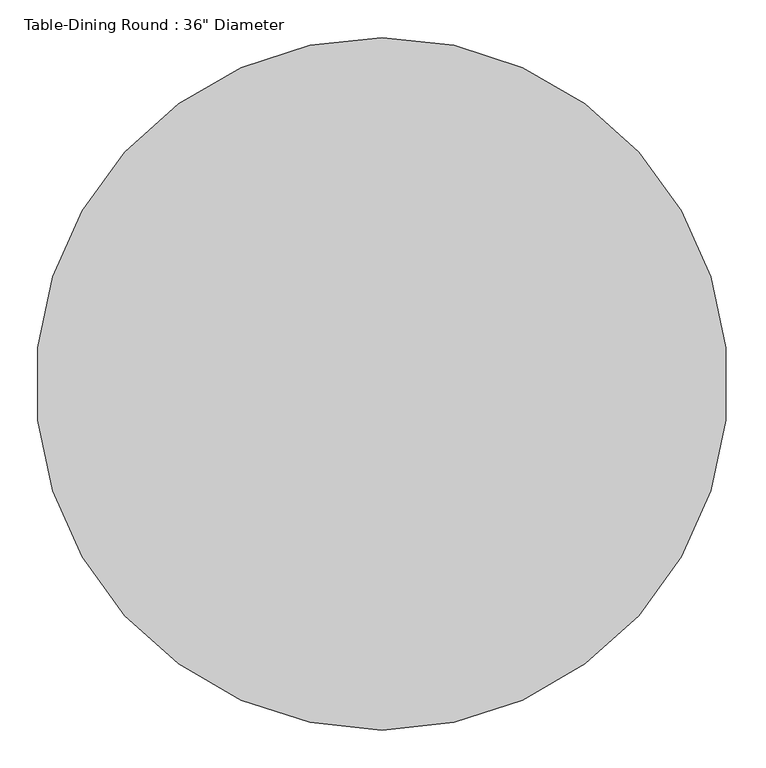
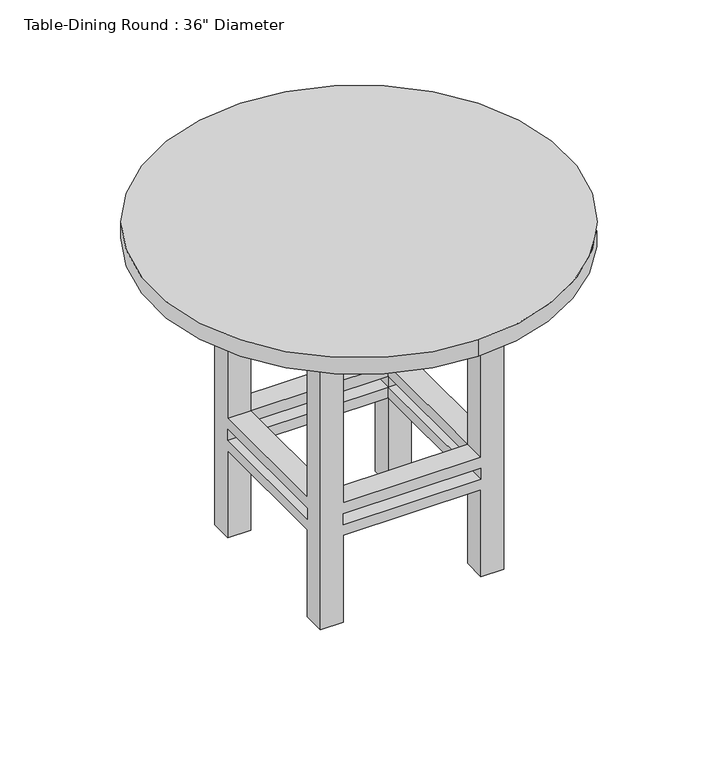
"""IFC4 building model written with IfcOpenShell, lengths in millimetres: furniture geometry."""

from ifc_helpers import new_model, si_unit, point, frame, frame_2d, origin, place, context, project, spatial, polyline, circle_curve, trimmed, segment, composite_curve, outline, extrude, faceted_brep, source, transform, mapped, element, save


def furniture_ec754799(model_context):
    return source(origin(), model_context, "Body", "SolidModel", [
        extrude(outline(polyline([(332.2819672, 43.7213115), (332.2819672, -413.4786885), (-124.9180328, -413.4786885), (-124.9180328, 43.7213115), (332.2819672, 43.7213115)]), holes=[polyline([(306.8819672, 18.3213115), (-99.5180328, 18.3213115), (-99.5180328, -388.0786885), (306.8819672, -388.0786885), (306.8819672, 18.3213115)])]), frame((0.0, 0.0, 647.7), z_axis=(0.0, 0.0, 1.0), x_axis=(1.0, 0.0, 0.0)), (0.0, 0.0, 1.0), 76.2),
        faceted_brep([(-48.7180328, 18.3213115, 723.9), (-99.5180328, 18.3213115, 723.9), (-99.5180328, -32.4786885, 723.9), (-48.7180328, -32.4786885, 723.9), (256.0819672, 18.3213115, 723.9), (256.0819672, -32.4786885, 723.9), (306.8819672, -32.4786885, 723.9), (306.8819672, 18.3213115, 723.9), (256.0819672, -388.0786885, 723.9), (306.8819672, -388.0786885, 723.9), (306.8819672, -337.2786885, 723.9), (256.0819672, -337.2786885, 723.9), (-48.7180328, -388.0786885, 723.9), (-48.7180328, -337.2786885, 723.9), (-99.5180328, -337.2786885, 723.9), (-99.5180328, -388.0786885, 723.9), (-48.7180328, 18.3213115, 0.0), (-48.7180328, -32.4786885, 0.0), (-99.5180328, -32.4786885, 0.0), (-99.5180328, 18.3213115, 0.0), (256.0819672, 18.3213115, 0.0), (306.8819672, 18.3213115, 0.0), (306.8819672, -32.4786885, 0.0), (256.0819672, -32.4786885, 0.0), (256.0819672, -388.0786885, 0.0), (256.0819672, -337.2786885, 0.0), (306.8819672, -337.2786885, 0.0), (306.8819672, -388.0786885, 0.0), (-48.7180328, -388.0786885, 0.0), (-99.5180328, -388.0786885, 0.0), (-99.5180328, -337.2786885, 0.0), (-48.7180328, -337.2786885, 0.0), (-48.7180328, 18.3213115, 279.4), (256.0819672, 18.3213115, 279.4), (256.0819672, 18.3213115, 203.2), (-48.7180328, 18.3213115, 203.2), (256.0819672, 18.3213115, 228.6), (256.0819672, 18.3213115, 254.0), (-48.7180328, 18.3213115, 254.0), (-48.7180328, 18.3213115, 228.6), (-99.5180328, -32.4786885, 203.2), (-99.5180328, -337.2786885, 203.2), (-99.5180328, -337.2786885, 279.4), (-99.5180328, -32.4786885, 279.4), (-99.5180328, -32.4786885, 228.6), (-99.5180328, -32.4786885, 254.0), (-99.5180328, -337.2786885, 254.0), (-99.5180328, -337.2786885, 228.6), (-48.7180328, -32.4786885, 279.4), (-48.7180328, -32.4786885, 203.2), (-48.7180328, -32.4786885, 228.6), (-48.7180328, -32.4786885, 254.0), (256.0819672, -32.4786885, 279.4), (256.0819672, -32.4786885, 203.2), (256.0819672, -32.4786885, 228.6), (256.0819672, -32.4786885, 254.0), (306.8819672, -32.4786885, 279.4), (306.8819672, -32.4786885, 203.2), (306.8819672, -32.4786885, 228.6), (306.8819672, -32.4786885, 254.0), (306.8819672, -337.2786885, 279.4), (306.8819672, -337.2786885, 203.2), (306.8819672, -337.2786885, 228.6), (306.8819672, -337.2786885, 254.0), (256.0819672, -388.0786885, 279.4), (-48.7180328, -388.0786885, 279.4), (-48.7180328, -388.0786885, 203.2), (256.0819672, -388.0786885, 203.2), (-48.7180328, -388.0786885, 228.6), (-48.7180328, -388.0786885, 254.0), (256.0819672, -388.0786885, 254.0), (256.0819672, -388.0786885, 228.6), (256.0819672, -337.2786885, 279.4), (256.0819672, -337.2786885, 203.2), (256.0819672, -337.2786885, 228.6), (256.0819672, -337.2786885, 254.0), (-48.7180328, -337.2786885, 279.4), (-48.7180328, -337.2786885, 203.2), (-48.7180328, -337.2786885, 228.6), (-48.7180328, -337.2786885, 254.0)], [[[0, 1, 2, 3]], [[4, 5, 6, 7]], [[8, 9, 10, 11]], [[12, 13, 14, 15]], [[16, 17, 18, 19]], [[20, 21, 22, 23]], [[24, 25, 26, 27]], [[28, 29, 30, 31]], [[1, 0, 32, 33, 4, 7, 21, 20, 34, 35, 16, 19], [36, 37, 38, 39]], [[2, 1, 19, 18, 40, 41, 30, 29, 15, 14, 42, 43], [44, 45, 46, 47]], [[3, 2, 43, 48]], [[18, 17, 49, 40]], [[44, 50, 51, 45]], [[0, 3, 48, 32]], [[17, 16, 35, 49]], [[50, 39, 38, 51]], [[5, 4, 33, 52]], [[20, 23, 53, 34]], [[36, 54, 55, 37]], [[6, 5, 52, 56]], [[23, 22, 57, 53]], [[54, 58, 59, 55]], [[21, 7, 6, 56, 60, 10, 9, 27, 26, 61, 57, 22], [62, 63, 59, 58]], [[27, 9, 8, 64, 65, 12, 15, 29, 28, 66, 67, 24], [68, 69, 70, 71]], [[11, 10, 60, 72]], [[26, 25, 73, 61]], [[62, 74, 75, 63]], [[8, 11, 72, 64]], [[25, 24, 67, 73]], [[74, 71, 70, 75]], [[13, 12, 65, 76]], [[28, 31, 77, 66]], [[68, 78, 79, 69]], [[14, 13, 76, 42]], [[31, 30, 41, 77]], [[78, 47, 46, 79]], [[54, 74, 62, 58]], [[74, 78, 68, 71]], [[78, 50, 44, 47]], [[50, 54, 36, 39]], [[53, 49, 35, 34]], [[49, 77, 41, 40]], [[77, 73, 67, 66]], [[73, 53, 57, 61]], [[74, 54, 53, 73]], [[78, 74, 73, 77]], [[50, 78, 77, 49]], [[54, 50, 49, 53]], [[52, 72, 60, 56]], [[72, 76, 65, 64]], [[76, 48, 43, 42]], [[48, 52, 33, 32]], [[55, 51, 38, 37]], [[51, 79, 46, 45]], [[79, 75, 70, 69]], [[75, 55, 59, 63]], [[72, 52, 55, 75]], [[76, 72, 75, 79]], [[48, 76, 79, 51]], [[52, 48, 51, 55]]]),
        extrude(outline(composite_curve([segment(trimmed(circle_curve(frame_2d((103.6819672, -184.8786885)), 457.2), [point((103.6819672, -642.0786885))], [point((103.6819672, 272.3213115))], False, "CARTESIAN"), True, "CONTINUOUS"), segment(trimmed(circle_curve(frame_2d((103.6819672, -184.8786885)), 457.2), [point((103.6819672, 272.3213115))], [point((103.6819672, -642.0786885))], False, "CARTESIAN"), True, "CONTINUOUS")], self_intersect=False)), frame((0.0, 0.0, 723.9), z_axis=(0.0, 0.0, 1.0), x_axis=(1.0, 0.0, 0.0)), (0.0, 0.0, 1.0), 38.1),
    ])


if __name__ == "__main__":
    model = new_model("IFC4")
    model_context = context("Model", 3, world=origin())
    ifc_project = project(units=[si_unit("LENGTHUNIT", "METRE", prefix="MILLI")], contexts=[model_context])
    site = spatial("IfcSite", under=ifc_project)
    building = spatial("IfcBuilding", under=site)
    placement = place(None, origin())
    furniture_shape = furniture_ec754799(model_context)
    element("IfcFurniture", 1, ObjectType="Table-Dining Round : 36\" Diameter", at=placement, inside=building, context=model_context, shape_type="MappedRepresentation", body=[
        mapped(furniture_shape, transform((0.0, 0.0, 0.0), x_axis=(1.0, 0.0, 0.0), y_axis=(0.0, 1.0, 0.0), z_axis=(0.0, 0.0, 1.0))),
    ])
    save(model, "model.ifc")

# Revit data of these elements
# Type "Table-Dining Round : 36\" Diameter"
#   Assembly Code = "E2020200"
#   Diameter = 914.4 mm
#   Height = 762 mm
#   Base Material = Pine
#   Top Material = Laminate, Linen, Matte
#   Default Elevation = 0
# Element 1 (IfcFurniture, "Table-Dining Round : 36\" Diameter")
#   Materials on its faces: "Pine", "Laminate, Linen, Matte"
# Materials
#   "Pine": class "Wood", colour RGB 223 192 134, transparency 0, Description = "Pinus Echinata", Cost = 0
#   "Laminate, Linen, Matte": class "Plastic", colour RGB 249 239 230, transparency 0, Description = "Plastic Laminate - Linen, Matte", Cost = 0
